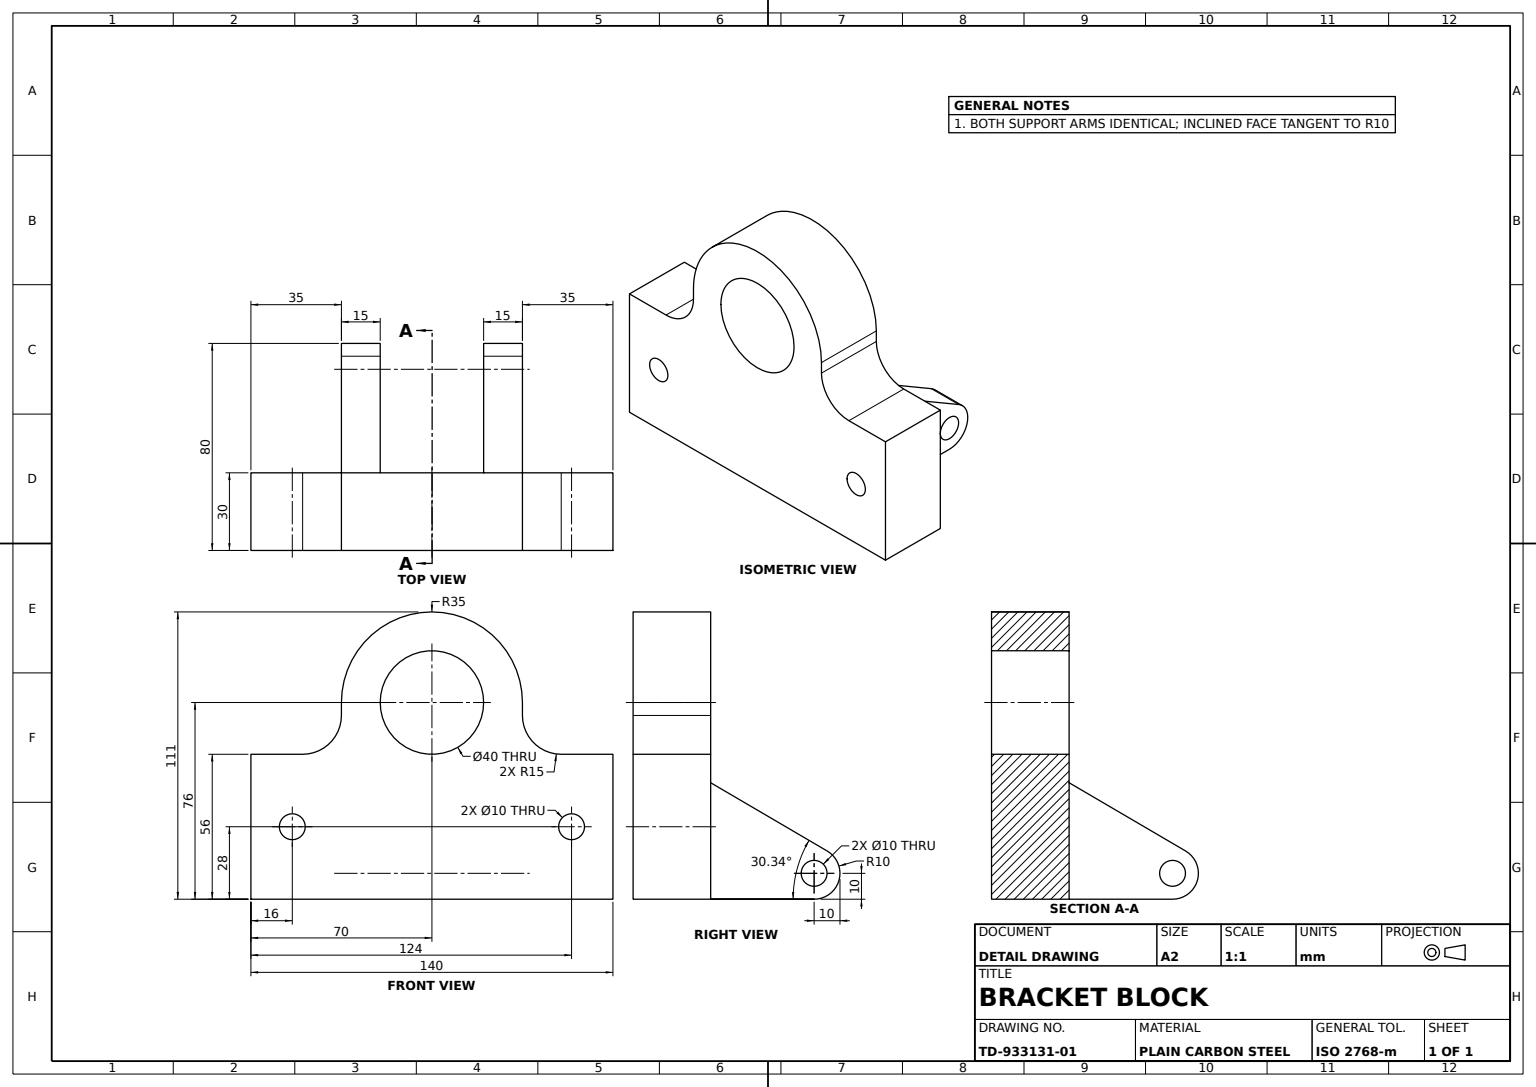
from build123d import *

# Parameters (mm, degrees)
BASE_PLATE_DEPTH         = 30
PIVOT_BORE_PROFILE_R     = 20
PIVOT_BORE_DEPTH         = 30
SUPPORT_ARM_DEPTH        = 15
PIVOT_LUG_DEPTH          = 15
LUG_HOLE_PROFILE_R       = 5
LUG_HOLE_DEPTH           = 70
MOUNTING_HOLES_PROFILE_R = 5
MOUNTING_HOLES_2X_DEPTH  = 70


with BuildPart() as part:
    # Base Plate Profile → Base Plate (new body)
    with BuildSketch(Plane.XY):
        with BuildLine():
            Line((0, 0), (0, 56))
            Line((0, 56), (20, 56))
            ThreePointArc((20, 56), (30.606601718, 60.393398282), (35, 71))
            Line((35, 71), (35, 76))
            ThreePointArc((35, 76), (70, 111), (105, 76))
            Line((105, 76), (105, 71))
            ThreePointArc((105, 71), (109.393398282, 60.393398282), (120, 56))
            Line((120, 56), (125, 56))
            Line((125, 56), (140, 56))
            Line((140, 56), (140, 0))
            Line((140, 0), (0, 0))
        make_face()
    extrude(amount=BASE_PLATE_DEPTH)

    # Pivot Bore Profile → Pivot Bore (cut)
    with BuildSketch(Plane.XY.offset(30)):
        with Locations((70, 76)):
            Circle(PIVOT_BORE_PROFILE_R)
    extrude(amount=-PIVOT_BORE_DEPTH, mode=Mode.SUBTRACT)

    # Support Arm Profile → Support Arm (add)
    with BuildSketch(Plane(origin=(35, 0, 0), x_dir=(0, 0, -1), z_dir=(1, 0, 0))):
        with BuildLine():
            Line((0, 0), (0, 45))
            Line((0, 45), (45.051517306, 18.630305493))
            ThreePointArc((45.051517306, 18.630305493), (49.651503897, 7.383041358), (40, 0))
            Line((40, 0), (0, 0))
        make_face()
    extrude(amount=SUPPORT_ARM_DEPTH)

    # Pivot Lug Profile → Pivot Lug (add)
    with BuildSketch(Plane(origin=(90, 0, 0), x_dir=(0, 0, -1), z_dir=(1, 0, 0))):
        with BuildLine():
            Line((0, 0), (0, 45))
            Line((0, 45), (45.051517306, 18.630305493))
            ThreePointArc((45.051517306, 18.630305493), (49.651503897, 7.383041358), (40, 0))
            Line((40, 0), (0, 0))
        make_face()
    extrude(amount=PIVOT_LUG_DEPTH)

    # Lug Hole Profile → Lug Hole (cut)
    with BuildSketch(Plane(origin=(105, 0, 0), x_dir=(0, 0, -1), z_dir=(1, 0, 0))):
        with Locations((40, 10)):
            Circle(LUG_HOLE_PROFILE_R)
    extrude(amount=-LUG_HOLE_DEPTH, mode=Mode.SUBTRACT)

    # Mounting Holes Profile → Mounting Holes 2x (cut)
    with BuildSketch(Plane(origin=(0, 0, 0), x_dir=(-1, 0, 0), z_dir=(0, 0, -1))):
        with Locations((-124, 28)):
            Circle(MOUNTING_HOLES_PROFILE_R)
        with Locations((-16, 28)):
            Circle(MOUNTING_HOLES_PROFILE_R)
    extrude(amount=-MOUNTING_HOLES_2X_DEPTH, mode=Mode.SUBTRACT)


solid = part.part
